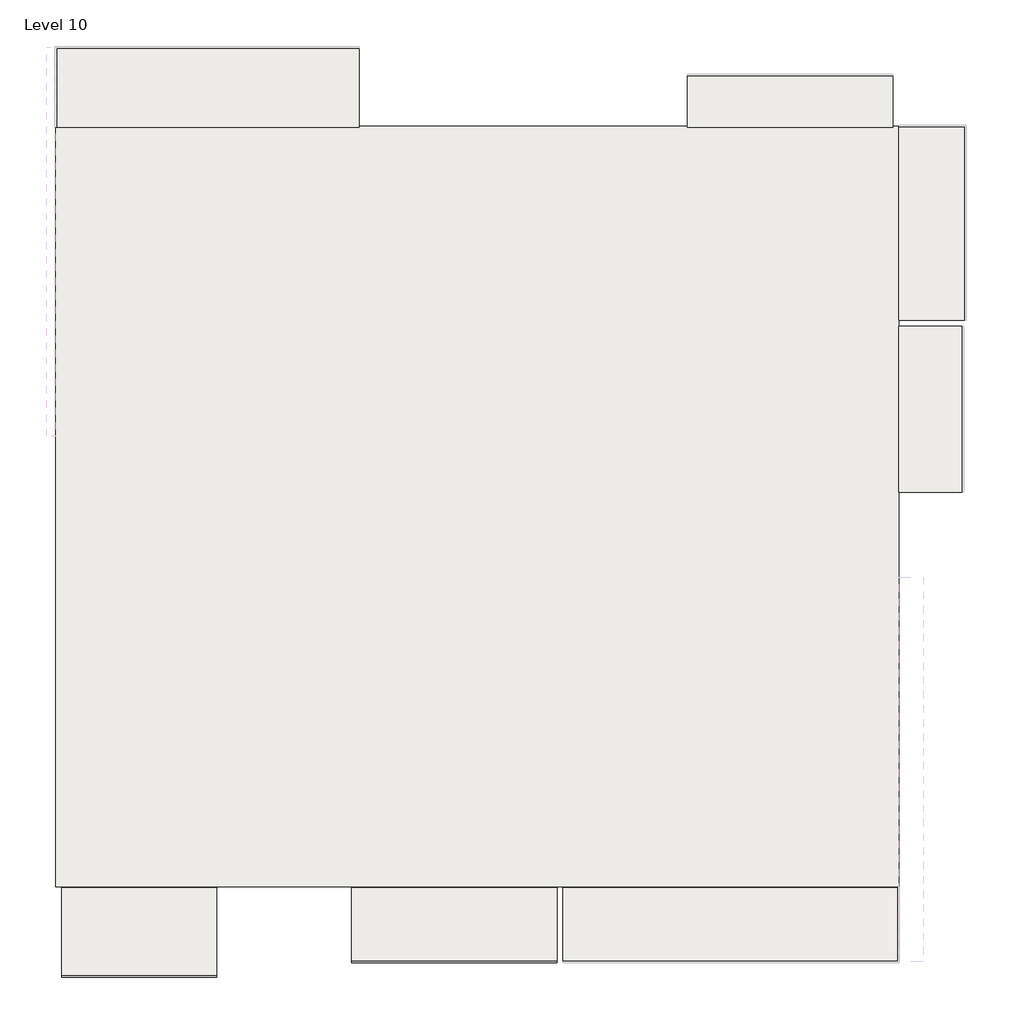
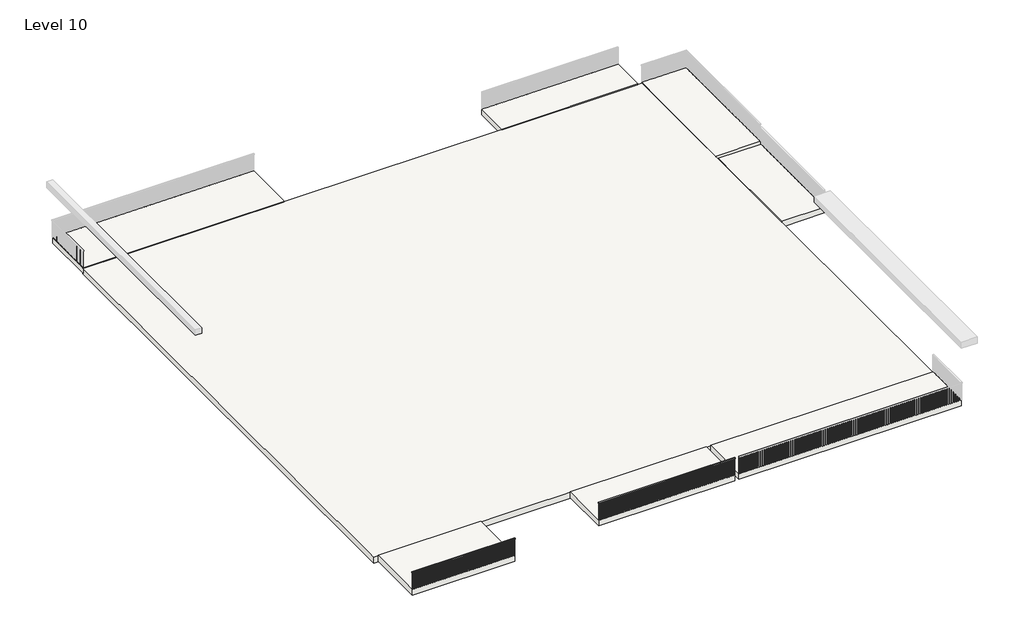
# One storey, part 1 of 5: 9 slabs, 2 railings.
"""IFC4 building model written with IfcOpenShell, lengths in millimetres."""

from ifc_helpers import new_model, si_unit, frame, origin, place, context, project, spatial, polyline, outline, extrude, element, save

model = new_model("IFC4")

# Units and contexts
model_context = context("Model", 3, world=origin())
ifc_project = project(units=[si_unit("LENGTHUNIT", "METRE", prefix="MILLI")], contexts=[model_context])

# Site, building, storey
site = spatial("IfcSite", under=ifc_project)
building = spatial("IfcBuilding", under=site)
storey = spatial("IfcBuildingStorey", under=building, Name="Level 10", Elevation=12496.8)

# Railings
placement = place(None, origin())
element("IfcRailing", 1, ObjectType="Handrail - Rectangular", at=placement, inside=storey, context=model_context, shape_type="SweptSolid", body=[
    extrude(outline(polyline([(-13630.2638778, -13399.9762475), (-13630.2638778, -13349.1762475), (-8499.4638778, -13349.1762475), (-8499.4638778, -13399.9762475), (-13630.2638778, -13399.9762475)])), frame((0.0, 0.0, 13360.4), z_axis=(0.0, 0.0, 1.0), x_axis=(1.0, 0.0, 0.0)), (0.0, 0.0, 1.0), 50.8),
    extrude(outline(polyline([(-8559.7888778, -13384.1012475), (-8559.7888778, -13365.0512475), (-8540.7388778, -13365.0512475), (-8540.7388778, -13384.1012475), (-8559.7888778, -13384.1012475)])), frame((0.0, 0.0, 12496.8), z_axis=(0.0, 0.0, 1.0), x_axis=(1.0, 0.0, 0.0)), (0.0, 0.0, 1.0), 863.6),
    extrude(outline(polyline([(-8661.3888778, -13384.1012475), (-8661.3888778, -13365.0512475), (-8642.3388778, -13365.0512475), (-8642.3388778, -13384.1012475), (-8661.3888778, -13384.1012475)])), frame((0.0, 0.0, 12496.8), z_axis=(0.0, 0.0, 1.0), x_axis=(1.0, 0.0, 0.0)), (0.0, 0.0, 1.0), 863.6),
    extrude(outline(polyline([(-8762.9888778, -13384.1012475), (-8762.9888778, -13365.0512475), (-8743.9388778, -13365.0512475), (-8743.9388778, -13384.1012475), (-8762.9888778, -13384.1012475)])), frame((0.0, 0.0, 12496.8), z_axis=(0.0, 0.0, 1.0), x_axis=(1.0, 0.0, 0.0)), (0.0, 0.0, 1.0), 863.6),
    extrude(outline(polyline([(-8864.5888778, -13384.1012475), (-8864.5888778, -13365.0512475), (-8845.5388778, -13365.0512475), (-8845.5388778, -13384.1012475), (-8864.5888778, -13384.1012475)])), frame((0.0, 0.0, 12496.8), z_axis=(0.0, 0.0, 1.0), x_axis=(1.0, 0.0, 0.0)), (0.0, 0.0, 1.0), 863.6),
    extrude(outline(polyline([(-8966.1888778, -13384.1012475), (-8966.1888778, -13365.0512475), (-8947.1388778, -13365.0512475), (-8947.1388778, -13384.1012475), (-8966.1888778, -13384.1012475)])), frame((0.0, 0.0, 12496.8), z_axis=(0.0, 0.0, 1.0), x_axis=(1.0, 0.0, 0.0)), (0.0, 0.0, 1.0), 863.6),
    extrude(outline(polyline([(-9067.7888778, -13384.1012475), (-9067.7888778, -13365.0512475), (-9048.7388778, -13365.0512475), (-9048.7388778, -13384.1012475), (-9067.7888778, -13384.1012475)])), frame((0.0, 0.0, 12496.8), z_axis=(0.0, 0.0, 1.0), x_axis=(1.0, 0.0, 0.0)), (0.0, 0.0, 1.0), 863.6),
    extrude(outline(polyline([(-9169.3888778, -13384.1012475), (-9169.3888778, -13365.0512475), (-9150.3388778, -13365.0512475), (-9150.3388778, -13384.1012475), (-9169.3888778, -13384.1012475)])), frame((0.0, 0.0, 12496.8), z_axis=(0.0, 0.0, 1.0), x_axis=(1.0, 0.0, 0.0)), (0.0, 0.0, 1.0), 863.6),
    extrude(outline(polyline([(-9270.9888778, -13384.1012475), (-9270.9888778, -13365.0512475), (-9251.9388778, -13365.0512475), (-9251.9388778, -13384.1012475), (-9270.9888778, -13384.1012475)])), frame((0.0, 0.0, 12496.8), z_axis=(0.0, 0.0, 1.0), x_axis=(1.0, 0.0, 0.0)), (0.0, 0.0, 1.0), 863.6),
    extrude(outline(polyline([(-9372.5888778, -13384.1012475), (-9372.5888778, -13365.0512475), (-9353.5388778, -13365.0512475), (-9353.5388778, -13384.1012475), (-9372.5888778, -13384.1012475)])), frame((0.0, 0.0, 12496.8), z_axis=(0.0, 0.0, 1.0), x_axis=(1.0, 0.0, 0.0)), (0.0, 0.0, 1.0), 863.6),
    extrude(outline(polyline([(-9474.1888778, -13384.1012475), (-9474.1888778, -13365.0512475), (-9455.1388778, -13365.0512475), (-9455.1388778, -13384.1012475), (-9474.1888778, -13384.1012475)])), frame((0.0, 0.0, 12496.8), z_axis=(0.0, 0.0, 1.0), x_axis=(1.0, 0.0, 0.0)), (0.0, 0.0, 1.0), 863.6),
    extrude(outline(polyline([(-9575.7888778, -13384.1012475), (-9575.7888778, -13365.0512475), (-9556.7388778, -13365.0512475), (-9556.7388778, -13384.1012475), (-9575.7888778, -13384.1012475)])), frame((0.0, 0.0, 12496.8), z_axis=(0.0, 0.0, 1.0), x_axis=(1.0, 0.0, 0.0)), (0.0, 0.0, 1.0), 863.6),
    extrude(outline(polyline([(-9677.3888778, -13384.1012475), (-9677.3888778, -13365.0512475), (-9658.3388778, -13365.0512475), (-9658.3388778, -13384.1012475), (-9677.3888778, -13384.1012475)])), frame((0.0, 0.0, 12496.8), z_axis=(0.0, 0.0, 1.0), x_axis=(1.0, 0.0, 0.0)), (0.0, 0.0, 1.0), 863.6),
    extrude(outline(polyline([(-9778.9888778, -13384.1012475), (-9778.9888778, -13365.0512475), (-9759.9388778, -13365.0512475), (-9759.9388778, -13384.1012475), (-9778.9888778, -13384.1012475)])), frame((0.0, 0.0, 12496.8), z_axis=(0.0, 0.0, 1.0), x_axis=(1.0, 0.0, 0.0)), (0.0, 0.0, 1.0), 863.6),
    extrude(outline(polyline([(-9880.5888778, -13384.1012475), (-9880.5888778, -13365.0512475), (-9861.5388778, -13365.0512475), (-9861.5388778, -13384.1012475), (-9880.5888778, -13384.1012475)])), frame((0.0, 0.0, 12496.8), z_axis=(0.0, 0.0, 1.0), x_axis=(1.0, 0.0, 0.0)), (0.0, 0.0, 1.0), 863.6),
    extrude(outline(polyline([(-9982.1888778, -13384.1012475), (-9982.1888778, -13365.0512475), (-9963.1388778, -13365.0512475), (-9963.1388778, -13384.1012475), (-9982.1888778, -13384.1012475)])), frame((0.0, 0.0, 12496.8), z_axis=(0.0, 0.0, 1.0), x_axis=(1.0, 0.0, 0.0)), (0.0, 0.0, 1.0), 863.6),
    extrude(outline(polyline([(-10083.7888778, -13384.1012475), (-10083.7888778, -13365.0512475), (-10064.7388778, -13365.0512475), (-10064.7388778, -13384.1012475), (-10083.7888778, -13384.1012475)])), frame((0.0, 0.0, 12496.8), z_axis=(0.0, 0.0, 1.0), x_axis=(1.0, 0.0, 0.0)), (0.0, 0.0, 1.0), 863.6),
    extrude(outline(polyline([(-10185.3888778, -13384.1012475), (-10185.3888778, -13365.0512475), (-10166.3388778, -13365.0512475), (-10166.3388778, -13384.1012475), (-10185.3888778, -13384.1012475)])), frame((0.0, 0.0, 12496.8), z_axis=(0.0, 0.0, 1.0), x_axis=(1.0, 0.0, 0.0)), (0.0, 0.0, 1.0), 863.6),
    extrude(outline(polyline([(-10286.9888778, -13384.1012475), (-10286.9888778, -13365.0512475), (-10267.9388778, -13365.0512475), (-10267.9388778, -13384.1012475), (-10286.9888778, -13384.1012475)])), frame((0.0, 0.0, 12496.8), z_axis=(0.0, 0.0, 1.0), x_axis=(1.0, 0.0, 0.0)), (0.0, 0.0, 1.0), 863.6),
    extrude(outline(polyline([(-10388.5888778, -13384.1012475), (-10388.5888778, -13365.0512475), (-10369.5388778, -13365.0512475), (-10369.5388778, -13384.1012475), (-10388.5888778, -13384.1012475)])), frame((0.0, 0.0, 12496.8), z_axis=(0.0, 0.0, 1.0), x_axis=(1.0, 0.0, 0.0)), (0.0, 0.0, 1.0), 863.6),
    extrude(outline(polyline([(-10490.1888778, -13384.1012475), (-10490.1888778, -13365.0512475), (-10471.1388778, -13365.0512475), (-10471.1388778, -13384.1012475), (-10490.1888778, -13384.1012475)])), frame((0.0, 0.0, 12496.8), z_axis=(0.0, 0.0, 1.0), x_axis=(1.0, 0.0, 0.0)), (0.0, 0.0, 1.0), 863.6),
    extrude(outline(polyline([(-10591.7888778, -13384.1012475), (-10591.7888778, -13365.0512475), (-10572.7388778, -13365.0512475), (-10572.7388778, -13384.1012475), (-10591.7888778, -13384.1012475)])), frame((0.0, 0.0, 12496.8), z_axis=(0.0, 0.0, 1.0), x_axis=(1.0, 0.0, 0.0)), (0.0, 0.0, 1.0), 863.6),
    extrude(outline(polyline([(-10693.3888778, -13384.1012475), (-10693.3888778, -13365.0512475), (-10674.3388778, -13365.0512475), (-10674.3388778, -13384.1012475), (-10693.3888778, -13384.1012475)])), frame((0.0, 0.0, 12496.8), z_axis=(0.0, 0.0, 1.0), x_axis=(1.0, 0.0, 0.0)), (0.0, 0.0, 1.0), 863.6),
    extrude(outline(polyline([(-10794.9888778, -13384.1012475), (-10794.9888778, -13365.0512475), (-10775.9388778, -13365.0512475), (-10775.9388778, -13384.1012475), (-10794.9888778, -13384.1012475)])), frame((0.0, 0.0, 12496.8), z_axis=(0.0, 0.0, 1.0), x_axis=(1.0, 0.0, 0.0)), (0.0, 0.0, 1.0), 863.6),
    extrude(outline(polyline([(-10896.5888778, -13384.1012475), (-10896.5888778, -13365.0512475), (-10877.5388778, -13365.0512475), (-10877.5388778, -13384.1012475), (-10896.5888778, -13384.1012475)])), frame((0.0, 0.0, 12496.8), z_axis=(0.0, 0.0, 1.0), x_axis=(1.0, 0.0, 0.0)), (0.0, 0.0, 1.0), 863.6),
    extrude(outline(polyline([(-10998.1888778, -13384.1012475), (-10998.1888778, -13365.0512475), (-10979.1388778, -13365.0512475), (-10979.1388778, -13384.1012475), (-10998.1888778, -13384.1012475)])), frame((0.0, 0.0, 12496.8), z_axis=(0.0, 0.0, 1.0), x_axis=(1.0, 0.0, 0.0)), (0.0, 0.0, 1.0), 863.6),
    extrude(outline(polyline([(-11099.7888778, -13384.1012475), (-11099.7888778, -13365.0512475), (-11080.7388778, -13365.0512475), (-11080.7388778, -13384.1012475), (-11099.7888778, -13384.1012475)])), frame((0.0, 0.0, 12496.8), z_axis=(0.0, 0.0, 1.0), x_axis=(1.0, 0.0, 0.0)), (0.0, 0.0, 1.0), 863.6),
    extrude(outline(polyline([(-11201.3888778, -13384.1012475), (-11201.3888778, -13365.0512475), (-11182.3388778, -13365.0512475), (-11182.3388778, -13384.1012475), (-11201.3888778, -13384.1012475)])), frame((0.0, 0.0, 12496.8), z_axis=(0.0, 0.0, 1.0), x_axis=(1.0, 0.0, 0.0)), (0.0, 0.0, 1.0), 863.6),
    extrude(outline(polyline([(-11302.9888778, -13384.1012475), (-11302.9888778, -13365.0512475), (-11283.9388778, -13365.0512475), (-11283.9388778, -13384.1012475), (-11302.9888778, -13384.1012475)])), frame((0.0, 0.0, 12496.8), z_axis=(0.0, 0.0, 1.0), x_axis=(1.0, 0.0, 0.0)), (0.0, 0.0, 1.0), 863.6),
    extrude(outline(polyline([(-11404.5888778, -13384.1012475), (-11404.5888778, -13365.0512475), (-11385.5388778, -13365.0512475), (-11385.5388778, -13384.1012475), (-11404.5888778, -13384.1012475)])), frame((0.0, 0.0, 12496.8), z_axis=(0.0, 0.0, 1.0), x_axis=(1.0, 0.0, 0.0)), (0.0, 0.0, 1.0), 863.6),
    extrude(outline(polyline([(-11506.1888778, -13384.1012475), (-11506.1888778, -13365.0512475), (-11487.1388778, -13365.0512475), (-11487.1388778, -13384.1012475), (-11506.1888778, -13384.1012475)])), frame((0.0, 0.0, 12496.8), z_axis=(0.0, 0.0, 1.0), x_axis=(1.0, 0.0, 0.0)), (0.0, 0.0, 1.0), 863.6),
    extrude(outline(polyline([(-11607.7888778, -13384.1012475), (-11607.7888778, -13365.0512475), (-11588.7388778, -13365.0512475), (-11588.7388778, -13384.1012475), (-11607.7888778, -13384.1012475)])), frame((0.0, 0.0, 12496.8), z_axis=(0.0, 0.0, 1.0), x_axis=(1.0, 0.0, 0.0)), (0.0, 0.0, 1.0), 863.6),
    extrude(outline(polyline([(-11709.3888778, -13384.1012475), (-11709.3888778, -13365.0512475), (-11690.3388778, -13365.0512475), (-11690.3388778, -13384.1012475), (-11709.3888778, -13384.1012475)])), frame((0.0, 0.0, 12496.8), z_axis=(0.0, 0.0, 1.0), x_axis=(1.0, 0.0, 0.0)), (0.0, 0.0, 1.0), 863.6),
    extrude(outline(polyline([(-11810.9888778, -13384.1012475), (-11810.9888778, -13365.0512475), (-11791.9388778, -13365.0512475), (-11791.9388778, -13384.1012475), (-11810.9888778, -13384.1012475)])), frame((0.0, 0.0, 12496.8), z_axis=(0.0, 0.0, 1.0), x_axis=(1.0, 0.0, 0.0)), (0.0, 0.0, 1.0), 863.6),
    extrude(outline(polyline([(-11912.5888778, -13384.1012475), (-11912.5888778, -13365.0512475), (-11893.5388778, -13365.0512475), (-11893.5388778, -13384.1012475), (-11912.5888778, -13384.1012475)])), frame((0.0, 0.0, 12496.8), z_axis=(0.0, 0.0, 1.0), x_axis=(1.0, 0.0, 0.0)), (0.0, 0.0, 1.0), 863.6),
    extrude(outline(polyline([(-12014.1888778, -13384.1012475), (-12014.1888778, -13365.0512475), (-11995.1388778, -13365.0512475), (-11995.1388778, -13384.1012475), (-12014.1888778, -13384.1012475)])), frame((0.0, 0.0, 12496.8), z_axis=(0.0, 0.0, 1.0), x_axis=(1.0, 0.0, 0.0)), (0.0, 0.0, 1.0), 863.6),
    extrude(outline(polyline([(-12115.7888778, -13384.1012475), (-12115.7888778, -13365.0512475), (-12096.7388778, -13365.0512475), (-12096.7388778, -13384.1012475), (-12115.7888778, -13384.1012475)])), frame((0.0, 0.0, 12496.8), z_axis=(0.0, 0.0, 1.0), x_axis=(1.0, 0.0, 0.0)), (0.0, 0.0, 1.0), 863.6),
    extrude(outline(polyline([(-12217.3888778, -13384.1012475), (-12217.3888778, -13365.0512475), (-12198.3388778, -13365.0512475), (-12198.3388778, -13384.1012475), (-12217.3888778, -13384.1012475)])), frame((0.0, 0.0, 12496.8), z_axis=(0.0, 0.0, 1.0), x_axis=(1.0, 0.0, 0.0)), (0.0, 0.0, 1.0), 863.6),
    extrude(outline(polyline([(-12318.9888778, -13384.1012475), (-12318.9888778, -13365.0512475), (-12299.9388778, -13365.0512475), (-12299.9388778, -13384.1012475), (-12318.9888778, -13384.1012475)])), frame((0.0, 0.0, 12496.8), z_axis=(0.0, 0.0, 1.0), x_axis=(1.0, 0.0, 0.0)), (0.0, 0.0, 1.0), 863.6),
    extrude(outline(polyline([(-12420.5888778, -13384.1012475), (-12420.5888778, -13365.0512475), (-12401.5388778, -13365.0512475), (-12401.5388778, -13384.1012475), (-12420.5888778, -13384.1012475)])), frame((0.0, 0.0, 12496.8), z_axis=(0.0, 0.0, 1.0), x_axis=(1.0, 0.0, 0.0)), (0.0, 0.0, 1.0), 863.6),
    extrude(outline(polyline([(-12522.1888778, -13384.1012475), (-12522.1888778, -13365.0512475), (-12503.1388778, -13365.0512475), (-12503.1388778, -13384.1012475), (-12522.1888778, -13384.1012475)])), frame((0.0, 0.0, 12496.8), z_axis=(0.0, 0.0, 1.0), x_axis=(1.0, 0.0, 0.0)), (0.0, 0.0, 1.0), 863.6),
    extrude(outline(polyline([(-12623.7888778, -13384.1012475), (-12623.7888778, -13365.0512475), (-12604.7388778, -13365.0512475), (-12604.7388778, -13384.1012475), (-12623.7888778, -13384.1012475)])), frame((0.0, 0.0, 12496.8), z_axis=(0.0, 0.0, 1.0), x_axis=(1.0, 0.0, 0.0)), (0.0, 0.0, 1.0), 863.6),
    extrude(outline(polyline([(-12725.3888778, -13384.1012475), (-12725.3888778, -13365.0512475), (-12706.3388778, -13365.0512475), (-12706.3388778, -13384.1012475), (-12725.3888778, -13384.1012475)])), frame((0.0, 0.0, 12496.8), z_axis=(0.0, 0.0, 1.0), x_axis=(1.0, 0.0, 0.0)), (0.0, 0.0, 1.0), 863.6),
    extrude(outline(polyline([(-12826.9888778, -13384.1012475), (-12826.9888778, -13365.0512475), (-12807.9388778, -13365.0512475), (-12807.9388778, -13384.1012475), (-12826.9888778, -13384.1012475)])), frame((0.0, 0.0, 12496.8), z_axis=(0.0, 0.0, 1.0), x_axis=(1.0, 0.0, 0.0)), (0.0, 0.0, 1.0), 863.6),
    extrude(outline(polyline([(-12928.5888778, -13384.1012475), (-12928.5888778, -13365.0512475), (-12909.5388778, -13365.0512475), (-12909.5388778, -13384.1012475), (-12928.5888778, -13384.1012475)])), frame((0.0, 0.0, 12496.8), z_axis=(0.0, 0.0, 1.0), x_axis=(1.0, 0.0, 0.0)), (0.0, 0.0, 1.0), 863.6),
    extrude(outline(polyline([(-13030.1888778, -13384.1012475), (-13030.1888778, -13365.0512475), (-13011.1388778, -13365.0512475), (-13011.1388778, -13384.1012475), (-13030.1888778, -13384.1012475)])), frame((0.0, 0.0, 12496.8), z_axis=(0.0, 0.0, 1.0), x_axis=(1.0, 0.0, 0.0)), (0.0, 0.0, 1.0), 863.6),
    extrude(outline(polyline([(-13131.7888778, -13384.1012475), (-13131.7888778, -13365.0512475), (-13112.7388778, -13365.0512475), (-13112.7388778, -13384.1012475), (-13131.7888778, -13384.1012475)])), frame((0.0, 0.0, 12496.8), z_axis=(0.0, 0.0, 1.0), x_axis=(1.0, 0.0, 0.0)), (0.0, 0.0, 1.0), 863.6),
    extrude(outline(polyline([(-13233.3888778, -13384.1012475), (-13233.3888778, -13365.0512475), (-13214.3388778, -13365.0512475), (-13214.3388778, -13384.1012475), (-13233.3888778, -13384.1012475)])), frame((0.0, 0.0, 12496.8), z_axis=(0.0, 0.0, 1.0), x_axis=(1.0, 0.0, 0.0)), (0.0, 0.0, 1.0), 863.6),
    extrude(outline(polyline([(-13334.9888778, -13384.1012475), (-13334.9888778, -13365.0512475), (-13315.9388778, -13365.0512475), (-13315.9388778, -13384.1012475), (-13334.9888778, -13384.1012475)])), frame((0.0, 0.0, 12496.8), z_axis=(0.0, 0.0, 1.0), x_axis=(1.0, 0.0, 0.0)), (0.0, 0.0, 1.0), 863.6),
    extrude(outline(polyline([(-13436.5888778, -13384.1012475), (-13436.5888778, -13365.0512475), (-13417.5388778, -13365.0512475), (-13417.5388778, -13384.1012475), (-13436.5888778, -13384.1012475)])), frame((0.0, 0.0, 12496.8), z_axis=(0.0, 0.0, 1.0), x_axis=(1.0, 0.0, 0.0)), (0.0, 0.0, 1.0), 863.6),
    extrude(outline(polyline([(-13538.1888778, -13384.1012475), (-13538.1888778, -13365.0512475), (-13519.1388778, -13365.0512475), (-13519.1388778, -13384.1012475), (-13538.1888778, -13384.1012475)])), frame((0.0, 0.0, 12496.8), z_axis=(0.0, 0.0, 1.0), x_axis=(1.0, 0.0, 0.0)), (0.0, 0.0, 1.0), 863.6),
    extrude(outline(polyline([(-8518.5138778, -13384.1012475), (-8518.5138778, -13365.0512475), (-8499.4638778, -13365.0512475), (-8499.4638778, -13384.1012475), (-8518.5138778, -13384.1012475)])), frame((0.0, 0.0, 12496.8), z_axis=(0.0, 0.0, 1.0), x_axis=(1.0, 0.0, 0.0)), (0.0, 0.0, 1.0), 863.6),
    extrude(outline(polyline([(-13630.2638778, -13384.1012475), (-13630.2638778, -13365.0512475), (-13611.2138778, -13365.0512475), (-13611.2138778, -13384.1012475), (-13630.2638778, -13384.1012475)])), frame((0.0, 0.0, 12496.8), z_axis=(0.0, 0.0, 1.0), x_axis=(1.0, 0.0, 0.0)), (0.0, 0.0, 1.0), 863.6),
])
element("IfcRailing", 2, ObjectType="Handrail - Rectangular", at=placement, inside=storey, context=model_context, shape_type="SweptSolid", body=[
    extrude(outline(polyline([(-4029.0638778, -12911.7749501), (-4029.0638778, -12860.9749501), (2778.1361222, -12860.9749501), (2778.1361222, -12911.7749501), (-4029.0638778, -12911.7749501)])), frame((0.0, 0.0, 13360.4), z_axis=(0.0, 0.0, 1.0), x_axis=(1.0, 0.0, 0.0)), (0.0, 0.0, 1.0), 50.8),
    extrude(outline(polyline([(2667.0111222, -12895.8999501), (2667.0111222, -12876.8499501), (2686.0611222, -12876.8499501), (2686.0611222, -12895.8999501), (2667.0111222, -12895.8999501)])), frame((0.0, 0.0, 12496.8), z_axis=(0.0, 0.0, 1.0), x_axis=(1.0, 0.0, 0.0)), (0.0, 0.0, 1.0), 863.6),
    extrude(outline(polyline([(2565.4111222, -12895.8999501), (2565.4111222, -12876.8499501), (2584.4611222, -12876.8499501), (2584.4611222, -12895.8999501), (2565.4111222, -12895.8999501)])), frame((0.0, 0.0, 12496.8), z_axis=(0.0, 0.0, 1.0), x_axis=(1.0, 0.0, 0.0)), (0.0, 0.0, 1.0), 863.6),
    extrude(outline(polyline([(2463.8111222, -12895.8999501), (2463.8111222, -12876.8499501), (2482.8611222, -12876.8499501), (2482.8611222, -12895.8999501), (2463.8111222, -12895.8999501)])), frame((0.0, 0.0, 12496.8), z_axis=(0.0, 0.0, 1.0), x_axis=(1.0, 0.0, 0.0)), (0.0, 0.0, 1.0), 863.6),
    extrude(outline(polyline([(2362.2111222, -12895.8999501), (2362.2111222, -12876.8499501), (2381.2611222, -12876.8499501), (2381.2611222, -12895.8999501), (2362.2111222, -12895.8999501)])), frame((0.0, 0.0, 12496.8), z_axis=(0.0, 0.0, 1.0), x_axis=(1.0, 0.0, 0.0)), (0.0, 0.0, 1.0), 863.6),
    extrude(outline(polyline([(2260.6111222, -12895.8999501), (2260.6111222, -12876.8499501), (2279.6611222, -12876.8499501), (2279.6611222, -12895.8999501), (2260.6111222, -12895.8999501)])), frame((0.0, 0.0, 12496.8), z_axis=(0.0, 0.0, 1.0), x_axis=(1.0, 0.0, 0.0)), (0.0, 0.0, 1.0), 863.6),
    extrude(outline(polyline([(2159.0111222, -12895.8999501), (2159.0111222, -12876.8499501), (2178.0611222, -12876.8499501), (2178.0611222, -12895.8999501), (2159.0111222, -12895.8999501)])), frame((0.0, 0.0, 12496.8), z_axis=(0.0, 0.0, 1.0), x_axis=(1.0, 0.0, 0.0)), (0.0, 0.0, 1.0), 863.6),
    extrude(outline(polyline([(2057.4111222, -12895.8999501), (2057.4111222, -12876.8499501), (2076.4611222, -12876.8499501), (2076.4611222, -12895.8999501), (2057.4111222, -12895.8999501)])), frame((0.0, 0.0, 12496.8), z_axis=(0.0, 0.0, 1.0), x_axis=(1.0, 0.0, 0.0)), (0.0, 0.0, 1.0), 863.6),
    extrude(outline(polyline([(1955.8111222, -12895.8999501), (1955.8111222, -12876.8499501), (1974.8611222, -12876.8499501), (1974.8611222, -12895.8999501), (1955.8111222, -12895.8999501)])), frame((0.0, 0.0, 12496.8), z_axis=(0.0, 0.0, 1.0), x_axis=(1.0, 0.0, 0.0)), (0.0, 0.0, 1.0), 863.6),
    extrude(outline(polyline([(1854.2111222, -12895.8999501), (1854.2111222, -12876.8499501), (1873.2611222, -12876.8499501), (1873.2611222, -12895.8999501), (1854.2111222, -12895.8999501)])), frame((0.0, 0.0, 12496.8), z_axis=(0.0, 0.0, 1.0), x_axis=(1.0, 0.0, 0.0)), (0.0, 0.0, 1.0), 863.6),
    extrude(outline(polyline([(1752.6111222, -12895.8999501), (1752.6111222, -12876.8499501), (1771.6611222, -12876.8499501), (1771.6611222, -12895.8999501), (1752.6111222, -12895.8999501)])), frame((0.0, 0.0, 12496.8), z_axis=(0.0, 0.0, 1.0), x_axis=(1.0, 0.0, 0.0)), (0.0, 0.0, 1.0), 863.6),
    extrude(outline(polyline([(1651.0111222, -12895.8999501), (1651.0111222, -12876.8499501), (1670.0611222, -12876.8499501), (1670.0611222, -12895.8999501), (1651.0111222, -12895.8999501)])), frame((0.0, 0.0, 12496.8), z_axis=(0.0, 0.0, 1.0), x_axis=(1.0, 0.0, 0.0)), (0.0, 0.0, 1.0), 863.6),
    extrude(outline(polyline([(1549.4111222, -12895.8999501), (1549.4111222, -12876.8499501), (1568.4611222, -12876.8499501), (1568.4611222, -12895.8999501), (1549.4111222, -12895.8999501)])), frame((0.0, 0.0, 12496.8), z_axis=(0.0, 0.0, 1.0), x_axis=(1.0, 0.0, 0.0)), (0.0, 0.0, 1.0), 863.6),
    extrude(outline(polyline([(1447.8111222, -12895.8999501), (1447.8111222, -12876.8499501), (1466.8611222, -12876.8499501), (1466.8611222, -12895.8999501), (1447.8111222, -12895.8999501)])), frame((0.0, 0.0, 12496.8), z_axis=(0.0, 0.0, 1.0), x_axis=(1.0, 0.0, 0.0)), (0.0, 0.0, 1.0), 863.6),
    extrude(outline(polyline([(1346.2111222, -12895.8999501), (1346.2111222, -12876.8499501), (1365.2611222, -12876.8499501), (1365.2611222, -12895.8999501), (1346.2111222, -12895.8999501)])), frame((0.0, 0.0, 12496.8), z_axis=(0.0, 0.0, 1.0), x_axis=(1.0, 0.0, 0.0)), (0.0, 0.0, 1.0), 863.6),
    extrude(outline(polyline([(1244.6111222, -12895.8999501), (1244.6111222, -12876.8499501), (1263.6611222, -12876.8499501), (1263.6611222, -12895.8999501), (1244.6111222, -12895.8999501)])), frame((0.0, 0.0, 12496.8), z_axis=(0.0, 0.0, 1.0), x_axis=(1.0, 0.0, 0.0)), (0.0, 0.0, 1.0), 863.6),
    extrude(outline(polyline([(1143.0111222, -12895.8999501), (1143.0111222, -12876.8499501), (1162.0611222, -12876.8499501), (1162.0611222, -12895.8999501), (1143.0111222, -12895.8999501)])), frame((0.0, 0.0, 12496.8), z_axis=(0.0, 0.0, 1.0), x_axis=(1.0, 0.0, 0.0)), (0.0, 0.0, 1.0), 863.6),
    extrude(outline(polyline([(1041.4111222, -12895.8999501), (1041.4111222, -12876.8499501), (1060.4611222, -12876.8499501), (1060.4611222, -12895.8999501), (1041.4111222, -12895.8999501)])), frame((0.0, 0.0, 12496.8), z_axis=(0.0, 0.0, 1.0), x_axis=(1.0, 0.0, 0.0)), (0.0, 0.0, 1.0), 863.6),
    extrude(outline(polyline([(939.8111222, -12895.8999501), (939.8111222, -12876.8499501), (958.8611222, -12876.8499501), (958.8611222, -12895.8999501), (939.8111222, -12895.8999501)])), frame((0.0, 0.0, 12496.8), z_axis=(0.0, 0.0, 1.0), x_axis=(1.0, 0.0, 0.0)), (0.0, 0.0, 1.0), 863.6),
    extrude(outline(polyline([(838.2111222, -12895.8999501), (838.2111222, -12876.8499501), (857.2611222, -12876.8499501), (857.2611222, -12895.8999501), (838.2111222, -12895.8999501)])), frame((0.0, 0.0, 12496.8), z_axis=(0.0, 0.0, 1.0), x_axis=(1.0, 0.0, 0.0)), (0.0, 0.0, 1.0), 863.6),
    extrude(outline(polyline([(736.6111222, -12895.8999501), (736.6111222, -12876.8499501), (755.6611222, -12876.8499501), (755.6611222, -12895.8999501), (736.6111222, -12895.8999501)])), frame((0.0, 0.0, 12496.8), z_axis=(0.0, 0.0, 1.0), x_axis=(1.0, 0.0, 0.0)), (0.0, 0.0, 1.0), 863.6),
    extrude(outline(polyline([(635.0111222, -12895.8999501), (635.0111222, -12876.8499501), (654.0611222, -12876.8499501), (654.0611222, -12895.8999501), (635.0111222, -12895.8999501)])), frame((0.0, 0.0, 12496.8), z_axis=(0.0, 0.0, 1.0), x_axis=(1.0, 0.0, 0.0)), (0.0, 0.0, 1.0), 863.6),
    extrude(outline(polyline([(533.4111222, -12895.8999501), (533.4111222, -12876.8499501), (552.4611222, -12876.8499501), (552.4611222, -12895.8999501), (533.4111222, -12895.8999501)])), frame((0.0, 0.0, 12496.8), z_axis=(0.0, 0.0, 1.0), x_axis=(1.0, 0.0, 0.0)), (0.0, 0.0, 1.0), 863.6),
    extrude(outline(polyline([(431.8111222, -12895.8999501), (431.8111222, -12876.8499501), (450.8611222, -12876.8499501), (450.8611222, -12895.8999501), (431.8111222, -12895.8999501)])), frame((0.0, 0.0, 12496.8), z_axis=(0.0, 0.0, 1.0), x_axis=(1.0, 0.0, 0.0)), (0.0, 0.0, 1.0), 863.6),
    extrude(outline(polyline([(330.2111222, -12895.8999501), (330.2111222, -12876.8499501), (349.2611222, -12876.8499501), (349.2611222, -12895.8999501), (330.2111222, -12895.8999501)])), frame((0.0, 0.0, 12496.8), z_axis=(0.0, 0.0, 1.0), x_axis=(1.0, 0.0, 0.0)), (0.0, 0.0, 1.0), 863.6),
    extrude(outline(polyline([(228.6111222, -12895.8999501), (228.6111222, -12876.8499501), (247.6611222, -12876.8499501), (247.6611222, -12895.8999501), (228.6111222, -12895.8999501)])), frame((0.0, 0.0, 12496.8), z_axis=(0.0, 0.0, 1.0), x_axis=(1.0, 0.0, 0.0)), (0.0, 0.0, 1.0), 863.6),
    extrude(outline(polyline([(127.0111222, -12895.8999501), (127.0111222, -12876.8499501), (146.0611222, -12876.8499501), (146.0611222, -12895.8999501), (127.0111222, -12895.8999501)])), frame((0.0, 0.0, 12496.8), z_axis=(0.0, 0.0, 1.0), x_axis=(1.0, 0.0, 0.0)), (0.0, 0.0, 1.0), 863.6),
    extrude(outline(polyline([(25.4111222, -12895.8999501), (25.4111222, -12876.8499501), (44.4611222, -12876.8499501), (44.4611222, -12895.8999501), (25.4111222, -12895.8999501)])), frame((0.0, 0.0, 12496.8), z_axis=(0.0, 0.0, 1.0), x_axis=(1.0, 0.0, 0.0)), (0.0, 0.0, 1.0), 863.6),
    extrude(outline(polyline([(-76.1888778, -12895.8999501), (-76.1888778, -12876.8499501), (-57.1388778, -12876.8499501), (-57.1388778, -12895.8999501), (-76.1888778, -12895.8999501)])), frame((0.0, 0.0, 12496.8), z_axis=(0.0, 0.0, 1.0), x_axis=(1.0, 0.0, 0.0)), (0.0, 0.0, 1.0), 863.6),
    extrude(outline(polyline([(-177.7888778, -12895.8999501), (-177.7888778, -12876.8499501), (-158.7388778, -12876.8499501), (-158.7388778, -12895.8999501), (-177.7888778, -12895.8999501)])), frame((0.0, 0.0, 12496.8), z_axis=(0.0, 0.0, 1.0), x_axis=(1.0, 0.0, 0.0)), (0.0, 0.0, 1.0), 863.6),
    extrude(outline(polyline([(-279.3888778, -12895.8999501), (-279.3888778, -12876.8499501), (-260.3388778, -12876.8499501), (-260.3388778, -12895.8999501), (-279.3888778, -12895.8999501)])), frame((0.0, 0.0, 12496.8), z_axis=(0.0, 0.0, 1.0), x_axis=(1.0, 0.0, 0.0)), (0.0, 0.0, 1.0), 863.6),
    extrude(outline(polyline([(-380.9888778, -12895.8999501), (-380.9888778, -12876.8499501), (-361.9388778, -12876.8499501), (-361.9388778, -12895.8999501), (-380.9888778, -12895.8999501)])), frame((0.0, 0.0, 12496.8), z_axis=(0.0, 0.0, 1.0), x_axis=(1.0, 0.0, 0.0)), (0.0, 0.0, 1.0), 863.6),
    extrude(outline(polyline([(-482.5888778, -12895.8999501), (-482.5888778, -12876.8499501), (-463.5388778, -12876.8499501), (-463.5388778, -12895.8999501), (-482.5888778, -12895.8999501)])), frame((0.0, 0.0, 12496.8), z_axis=(0.0, 0.0, 1.0), x_axis=(1.0, 0.0, 0.0)), (0.0, 0.0, 1.0), 863.6),
    extrude(outline(polyline([(-584.1888778, -12895.8999501), (-584.1888778, -12876.8499501), (-565.1388778, -12876.8499501), (-565.1388778, -12895.8999501), (-584.1888778, -12895.8999501)])), frame((0.0, 0.0, 12496.8), z_axis=(0.0, 0.0, 1.0), x_axis=(1.0, 0.0, 0.0)), (0.0, 0.0, 1.0), 863.6),
    extrude(outline(polyline([(-685.7888778, -12895.8999501), (-685.7888778, -12876.8499501), (-666.7388778, -12876.8499501), (-666.7388778, -12895.8999501), (-685.7888778, -12895.8999501)])), frame((0.0, 0.0, 12496.8), z_axis=(0.0, 0.0, 1.0), x_axis=(1.0, 0.0, 0.0)), (0.0, 0.0, 1.0), 863.6),
    extrude(outline(polyline([(-787.3888778, -12895.8999501), (-787.3888778, -12876.8499501), (-768.3388778, -12876.8499501), (-768.3388778, -12895.8999501), (-787.3888778, -12895.8999501)])), frame((0.0, 0.0, 12496.8), z_axis=(0.0, 0.0, 1.0), x_axis=(1.0, 0.0, 0.0)), (0.0, 0.0, 1.0), 863.6),
    extrude(outline(polyline([(-888.9888778, -12895.8999501), (-888.9888778, -12876.8499501), (-869.9388778, -12876.8499501), (-869.9388778, -12895.8999501), (-888.9888778, -12895.8999501)])), frame((0.0, 0.0, 12496.8), z_axis=(0.0, 0.0, 1.0), x_axis=(1.0, 0.0, 0.0)), (0.0, 0.0, 1.0), 863.6),
    extrude(outline(polyline([(-990.5888778, -12895.8999501), (-990.5888778, -12876.8499501), (-971.5388778, -12876.8499501), (-971.5388778, -12895.8999501), (-990.5888778, -12895.8999501)])), frame((0.0, 0.0, 12496.8), z_axis=(0.0, 0.0, 1.0), x_axis=(1.0, 0.0, 0.0)), (0.0, 0.0, 1.0), 863.6),
    extrude(outline(polyline([(-1092.1888778, -12895.8999501), (-1092.1888778, -12876.8499501), (-1073.1388778, -12876.8499501), (-1073.1388778, -12895.8999501), (-1092.1888778, -12895.8999501)])), frame((0.0, 0.0, 12496.8), z_axis=(0.0, 0.0, 1.0), x_axis=(1.0, 0.0, 0.0)), (0.0, 0.0, 1.0), 863.6),
    extrude(outline(polyline([(-1193.7888778, -12895.8999501), (-1193.7888778, -12876.8499501), (-1174.7388778, -12876.8499501), (-1174.7388778, -12895.8999501), (-1193.7888778, -12895.8999501)])), frame((0.0, 0.0, 12496.8), z_axis=(0.0, 0.0, 1.0), x_axis=(1.0, 0.0, 0.0)), (0.0, 0.0, 1.0), 863.6),
    extrude(outline(polyline([(-1295.3888778, -12895.8999501), (-1295.3888778, -12876.8499501), (-1276.3388778, -12876.8499501), (-1276.3388778, -12895.8999501), (-1295.3888778, -12895.8999501)])), frame((0.0, 0.0, 12496.8), z_axis=(0.0, 0.0, 1.0), x_axis=(1.0, 0.0, 0.0)), (0.0, 0.0, 1.0), 863.6),
    extrude(outline(polyline([(-1396.9888778, -12895.8999501), (-1396.9888778, -12876.8499501), (-1377.9388778, -12876.8499501), (-1377.9388778, -12895.8999501), (-1396.9888778, -12895.8999501)])), frame((0.0, 0.0, 12496.8), z_axis=(0.0, 0.0, 1.0), x_axis=(1.0, 0.0, 0.0)), (0.0, 0.0, 1.0), 863.6),
    extrude(outline(polyline([(-1498.5888778, -12895.8999501), (-1498.5888778, -12876.8499501), (-1479.5388778, -12876.8499501), (-1479.5388778, -12895.8999501), (-1498.5888778, -12895.8999501)])), frame((0.0, 0.0, 12496.8), z_axis=(0.0, 0.0, 1.0), x_axis=(1.0, 0.0, 0.0)), (0.0, 0.0, 1.0), 863.6),
    extrude(outline(polyline([(-1600.1888778, -12895.8999501), (-1600.1888778, -12876.8499501), (-1581.1388778, -12876.8499501), (-1581.1388778, -12895.8999501), (-1600.1888778, -12895.8999501)])), frame((0.0, 0.0, 12496.8), z_axis=(0.0, 0.0, 1.0), x_axis=(1.0, 0.0, 0.0)), (0.0, 0.0, 1.0), 863.6),
    extrude(outline(polyline([(-1701.7888778, -12895.8999501), (-1701.7888778, -12876.8499501), (-1682.7388778, -12876.8499501), (-1682.7388778, -12895.8999501), (-1701.7888778, -12895.8999501)])), frame((0.0, 0.0, 12496.8), z_axis=(0.0, 0.0, 1.0), x_axis=(1.0, 0.0, 0.0)), (0.0, 0.0, 1.0), 863.6),
    extrude(outline(polyline([(-1803.3888778, -12895.8999501), (-1803.3888778, -12876.8499501), (-1784.3388778, -12876.8499501), (-1784.3388778, -12895.8999501), (-1803.3888778, -12895.8999501)])), frame((0.0, 0.0, 12496.8), z_axis=(0.0, 0.0, 1.0), x_axis=(1.0, 0.0, 0.0)), (0.0, 0.0, 1.0), 863.6),
    extrude(outline(polyline([(-1904.9888778, -12895.8999501), (-1904.9888778, -12876.8499501), (-1885.9388778, -12876.8499501), (-1885.9388778, -12895.8999501), (-1904.9888778, -12895.8999501)])), frame((0.0, 0.0, 12496.8), z_axis=(0.0, 0.0, 1.0), x_axis=(1.0, 0.0, 0.0)), (0.0, 0.0, 1.0), 863.6),
    extrude(outline(polyline([(-2006.5888778, -12895.8999501), (-2006.5888778, -12876.8499501), (-1987.5388778, -12876.8499501), (-1987.5388778, -12895.8999501), (-2006.5888778, -12895.8999501)])), frame((0.0, 0.0, 12496.8), z_axis=(0.0, 0.0, 1.0), x_axis=(1.0, 0.0, 0.0)), (0.0, 0.0, 1.0), 863.6),
    extrude(outline(polyline([(-2108.1888778, -12895.8999501), (-2108.1888778, -12876.8499501), (-2089.1388778, -12876.8499501), (-2089.1388778, -12895.8999501), (-2108.1888778, -12895.8999501)])), frame((0.0, 0.0, 12496.8), z_axis=(0.0, 0.0, 1.0), x_axis=(1.0, 0.0, 0.0)), (0.0, 0.0, 1.0), 863.6),
    extrude(outline(polyline([(-2209.7888778, -12895.8999501), (-2209.7888778, -12876.8499501), (-2190.7388778, -12876.8499501), (-2190.7388778, -12895.8999501), (-2209.7888778, -12895.8999501)])), frame((0.0, 0.0, 12496.8), z_axis=(0.0, 0.0, 1.0), x_axis=(1.0, 0.0, 0.0)), (0.0, 0.0, 1.0), 863.6),
    extrude(outline(polyline([(-2311.3888778, -12895.8999501), (-2311.3888778, -12876.8499501), (-2292.3388778, -12876.8499501), (-2292.3388778, -12895.8999501), (-2311.3888778, -12895.8999501)])), frame((0.0, 0.0, 12496.8), z_axis=(0.0, 0.0, 1.0), x_axis=(1.0, 0.0, 0.0)), (0.0, 0.0, 1.0), 863.6),
    extrude(outline(polyline([(-2412.9888778, -12895.8999501), (-2412.9888778, -12876.8499501), (-2393.9388778, -12876.8499501), (-2393.9388778, -12895.8999501), (-2412.9888778, -12895.8999501)])), frame((0.0, 0.0, 12496.8), z_axis=(0.0, 0.0, 1.0), x_axis=(1.0, 0.0, 0.0)), (0.0, 0.0, 1.0), 863.6),
    extrude(outline(polyline([(-2514.5888778, -12895.8999501), (-2514.5888778, -12876.8499501), (-2495.5388778, -12876.8499501), (-2495.5388778, -12895.8999501), (-2514.5888778, -12895.8999501)])), frame((0.0, 0.0, 12496.8), z_axis=(0.0, 0.0, 1.0), x_axis=(1.0, 0.0, 0.0)), (0.0, 0.0, 1.0), 863.6),
    extrude(outline(polyline([(-2616.1888778, -12895.8999501), (-2616.1888778, -12876.8499501), (-2597.1388778, -12876.8499501), (-2597.1388778, -12895.8999501), (-2616.1888778, -12895.8999501)])), frame((0.0, 0.0, 12496.8), z_axis=(0.0, 0.0, 1.0), x_axis=(1.0, 0.0, 0.0)), (0.0, 0.0, 1.0), 863.6),
    extrude(outline(polyline([(-2717.7888778, -12895.8999501), (-2717.7888778, -12876.8499501), (-2698.7388778, -12876.8499501), (-2698.7388778, -12895.8999501), (-2717.7888778, -12895.8999501)])), frame((0.0, 0.0, 12496.8), z_axis=(0.0, 0.0, 1.0), x_axis=(1.0, 0.0, 0.0)), (0.0, 0.0, 1.0), 863.6),
    extrude(outline(polyline([(-2819.3888778, -12895.8999501), (-2819.3888778, -12876.8499501), (-2800.3388778, -12876.8499501), (-2800.3388778, -12895.8999501), (-2819.3888778, -12895.8999501)])), frame((0.0, 0.0, 12496.8), z_axis=(0.0, 0.0, 1.0), x_axis=(1.0, 0.0, 0.0)), (0.0, 0.0, 1.0), 863.6),
    extrude(outline(polyline([(-2920.9888778, -12895.8999501), (-2920.9888778, -12876.8499501), (-2901.9388778, -12876.8499501), (-2901.9388778, -12895.8999501), (-2920.9888778, -12895.8999501)])), frame((0.0, 0.0, 12496.8), z_axis=(0.0, 0.0, 1.0), x_axis=(1.0, 0.0, 0.0)), (0.0, 0.0, 1.0), 863.6),
    extrude(outline(polyline([(-3022.5888778, -12895.8999501), (-3022.5888778, -12876.8499501), (-3003.5388778, -12876.8499501), (-3003.5388778, -12895.8999501), (-3022.5888778, -12895.8999501)])), frame((0.0, 0.0, 12496.8), z_axis=(0.0, 0.0, 1.0), x_axis=(1.0, 0.0, 0.0)), (0.0, 0.0, 1.0), 863.6),
    extrude(outline(polyline([(-3124.1888778, -12895.8999501), (-3124.1888778, -12876.8499501), (-3105.1388778, -12876.8499501), (-3105.1388778, -12895.8999501), (-3124.1888778, -12895.8999501)])), frame((0.0, 0.0, 12496.8), z_axis=(0.0, 0.0, 1.0), x_axis=(1.0, 0.0, 0.0)), (0.0, 0.0, 1.0), 863.6),
    extrude(outline(polyline([(-3225.7888778, -12895.8999501), (-3225.7888778, -12876.8499501), (-3206.7388778, -12876.8499501), (-3206.7388778, -12895.8999501), (-3225.7888778, -12895.8999501)])), frame((0.0, 0.0, 12496.8), z_axis=(0.0, 0.0, 1.0), x_axis=(1.0, 0.0, 0.0)), (0.0, 0.0, 1.0), 863.6),
    extrude(outline(polyline([(-3327.3888778, -12895.8999501), (-3327.3888778, -12876.8499501), (-3308.3388778, -12876.8499501), (-3308.3388778, -12895.8999501), (-3327.3888778, -12895.8999501)])), frame((0.0, 0.0, 12496.8), z_axis=(0.0, 0.0, 1.0), x_axis=(1.0, 0.0, 0.0)), (0.0, 0.0, 1.0), 863.6),
    extrude(outline(polyline([(-3428.9888778, -12895.8999501), (-3428.9888778, -12876.8499501), (-3409.9388778, -12876.8499501), (-3409.9388778, -12895.8999501), (-3428.9888778, -12895.8999501)])), frame((0.0, 0.0, 12496.8), z_axis=(0.0, 0.0, 1.0), x_axis=(1.0, 0.0, 0.0)), (0.0, 0.0, 1.0), 863.6),
    extrude(outline(polyline([(-3530.5888778, -12895.8999501), (-3530.5888778, -12876.8499501), (-3511.5388778, -12876.8499501), (-3511.5388778, -12895.8999501), (-3530.5888778, -12895.8999501)])), frame((0.0, 0.0, 12496.8), z_axis=(0.0, 0.0, 1.0), x_axis=(1.0, 0.0, 0.0)), (0.0, 0.0, 1.0), 863.6),
    extrude(outline(polyline([(-3632.1888778, -12895.8999501), (-3632.1888778, -12876.8499501), (-3613.1388778, -12876.8499501), (-3613.1388778, -12895.8999501), (-3632.1888778, -12895.8999501)])), frame((0.0, 0.0, 12496.8), z_axis=(0.0, 0.0, 1.0), x_axis=(1.0, 0.0, 0.0)), (0.0, 0.0, 1.0), 863.6),
    extrude(outline(polyline([(-3733.7888778, -12895.8999501), (-3733.7888778, -12876.8499501), (-3714.7388778, -12876.8499501), (-3714.7388778, -12895.8999501), (-3733.7888778, -12895.8999501)])), frame((0.0, 0.0, 12496.8), z_axis=(0.0, 0.0, 1.0), x_axis=(1.0, 0.0, 0.0)), (0.0, 0.0, 1.0), 863.6),
    extrude(outline(polyline([(-3835.3888778, -12895.8999501), (-3835.3888778, -12876.8499501), (-3816.3388778, -12876.8499501), (-3816.3388778, -12895.8999501), (-3835.3888778, -12895.8999501)])), frame((0.0, 0.0, 12496.8), z_axis=(0.0, 0.0, 1.0), x_axis=(1.0, 0.0, 0.0)), (0.0, 0.0, 1.0), 863.6),
    extrude(outline(polyline([(-3936.9888778, -12895.8999501), (-3936.9888778, -12876.8499501), (-3917.9388778, -12876.8499501), (-3917.9388778, -12895.8999501), (-3936.9888778, -12895.8999501)])), frame((0.0, 0.0, 12496.8), z_axis=(0.0, 0.0, 1.0), x_axis=(1.0, 0.0, 0.0)), (0.0, 0.0, 1.0), 863.6),
    extrude(outline(polyline([(2759.0861222, -12895.8999501), (2759.0861222, -12876.8499501), (2778.1361222, -12876.8499501), (2778.1361222, -12895.8999501), (2759.0861222, -12895.8999501)])), frame((0.0, 0.0, 12496.8), z_axis=(0.0, 0.0, 1.0), x_axis=(1.0, 0.0, 0.0)), (0.0, 0.0, 1.0), 863.6),
    extrude(outline(polyline([(-4029.0638778, -12895.8999501), (-4029.0638778, -12876.8499501), (-4010.0138778, -12876.8499501), (-4010.0138778, -12895.8999501), (-4029.0638778, -12895.8999501)])), frame((0.0, 0.0, 12496.8), z_axis=(0.0, 0.0, 1.0), x_axis=(1.0, 0.0, 0.0)), (0.0, 0.0, 1.0), 863.6),
])

# Slabs
element("IfcSlab", 3, at=placement, inside=storey, context=model_context, shape_type="SweptSolid", body=[
    extrude(outline(polyline([(14106.5361222, -10428.1762475), (14106.5361222, -12886.3749501), (2981.3361222, -12886.3749501), (2981.3361222, -10428.1762475), (14106.5361222, -10428.1762475)])), frame((0.0, 0.0, 12192.0), z_axis=(0.0, 0.0, 1.0), x_axis=(1.0, 0.0, 0.0)), (0.0, 0.0, 1.0), 304.8),
])
element("IfcSlab", 4, at=placement, inside=storey, context=model_context, shape_type="SweptSolid", body=[
    extrude(outline(polyline([(-8499.4638778, -10428.1762475), (-8499.4638778, -13374.5762475), (-13630.2638778, -13374.5762475), (-13630.2638778, -10428.1762475), (-8499.4638778, -10428.1762475)])), frame((0.0, 0.0, 12192.0), z_axis=(0.0, 0.0, 1.0), x_axis=(1.0, 0.0, 0.0)), (0.0, 0.0, 1.0), 304.8),
])
element("IfcSlab", 5, at=placement, inside=storey, context=model_context, shape_type="SweptSolid", body=[
    extrude(outline(polyline([(2778.1361222, -10428.1762475), (2778.1361222, -12886.3749501), (-4029.0638778, -12886.3749501), (-4029.0638778, -10428.1762475), (2778.1361222, -10428.1762475)])), frame((0.0, 0.0, 12192.0), z_axis=(0.0, 0.0, 1.0), x_axis=(1.0, 0.0, 0.0)), (0.0, 0.0, 1.0), 304.8),
])
element("IfcSlab", 6, at=placement, inside=storey, context=model_context, shape_type="SweptSolid", body=[
    extrude(outline(polyline([(16240.1361222, 8164.6237525), (16240.1361222, 2678.2237525), (14106.5361222, 2678.2237525), (14106.5361222, 8164.6237525), (16240.1361222, 8164.6237525)])), frame((0.0, 0.0, 12192.0), z_axis=(0.0, 0.0, 1.0), x_axis=(1.0, 0.0, 0.0)), (0.0, 0.0, 1.0), 304.8),
])
element("IfcSlab", 7, at=placement, inside=storey, context=model_context, shape_type="SweptSolid", body=[
    extrude(outline(polyline([(16321.4289933, 14798.144107), (16321.4289933, 8367.8237525), (14106.5361222, 8367.8237525), (14106.5361222, 14798.144107), (16321.4289933, 14798.144107)])), frame((0.0, 0.0, 12192.0), z_axis=(0.0, 0.0, 1.0), x_axis=(1.0, 0.0, 0.0)), (0.0, 0.0, 1.0), 304.8),
])
element("IfcSlab", 8, at=placement, inside=storey, context=model_context, shape_type="SweptSolid", body=[
    extrude(outline(polyline([(13903.3361222, 14768.6237525), (7096.1361222, 14768.6237525), (7096.1361222, 16495.8237525), (13903.3361222, 16495.8237525), (13903.3361222, 14768.6237525)])), frame((0.0, 0.0, 12192.0), z_axis=(0.0, 0.0, 1.0), x_axis=(1.0, 0.0, 0.0)), (0.0, 0.0, 1.0), 304.8),
])
element("IfcSlab", 9, at=placement, inside=storey, context=model_context, shape_type="SweptSolid", body=[
    extrude(outline(polyline([(-13833.4638778, 14768.6237525), (-13833.4638778, 17410.2237525), (-3775.0638778, 17410.2237525), (-3775.0638778, 14768.6237525), (-13833.4638778, 14768.6237525)])), frame((0.0, 0.0, 12192.0), z_axis=(0.0, 0.0, 1.0), x_axis=(1.0, 0.0, 0.0)), (0.0, 0.0, 1.0), 304.8),
])
element("IfcSlab", 10, ObjectType="Generic - 12\"", at=placement, inside=storey, context=model_context, shape_type="SweptSolid", body=[
    extrude(outline(polyline([(14106.5361222, 14798.144107), (14106.5361222, -10398.655893), (-13833.4638778, -10398.655893), (-13833.4638778, 14798.144107), (14106.5361222, 14798.144107)])), frame((0.0, 0.0, 12145.6940312), z_axis=(0.0, 0.0, 1.0), x_axis=(1.0, 0.0, 0.0)), (0.0, 0.0, 1.0), 304.8),
])
element("IfcSlab", 11, ObjectType="Generic - 12\"", at=placement, inside=storey, context=model_context, shape_type="SweptSolid", body=[
    extrude(outline(polyline([(16240.1361222, 8164.6237525), (16240.1361222, 2678.2237525), (14106.5361222, 2678.2237525), (14106.5361222, 8164.6237525), (16240.1361222, 8164.6237525)])), frame((0.0, 0.0, 12192.0), z_axis=(0.0, 0.0, 1.0), x_axis=(1.0, 0.0, 0.0)), (0.0, 0.0, 1.0), 304.8),
])

save(model, "model.ifc")

# Revit data of these elements
# Type "Handrail - Rectangular"
#   Assembly Code = "C2010400"
#   built-in parameter 1008612 = 0.0416667 (stored number, unit not read)
#   built-in parameter 1008611 = 0.0416667 (stored number, unit not read)
#   built-in parameter 1008609 = 0.333333 (stored number, unit not read)
#   built-in parameter 1008604 = 0.166667 (stored number, unit not read)
#   built-in parameter 1008603 = 0.166667 (stored number, unit not read)
#   Railing Height = 3' - 0"
#   built-in parameter 1008630 = 2
#   built-in parameter 1008610 = 2
#   built-in parameter 1008618 = Baluster - Square : 3/4"
# Type
#   Assembly Code = "B1010"
#   Function = 0
#   Layers, outside or top first: 1' - 0" "Tile, Porcelain, 4in" (function 1)
# Type "Generic - 12\""
#   Assembly Code = "B1010"
#   Function = 0
#   Layers, outside or top first: 1' - 0" no material (function 1)
# Elements 1, 2 (IfcRailing, "Handrail - Rectangular")
#   Phase Created = New Construction
# Elements 3, 4, 5, 6, 7, 8 (IfcSlab)
#   Height Offset From Level = 0' - 0"
#   Phase Created = New Construction
#   Materials on its faces: "Tile, Porcelain, 4in"
# Element 9 (IfcSlab)
#   built-in parameter 1001955 = 3.14159 (stored number, unit not read)
#   Height Offset From Level = 0' - 0"
#   Phase Created = New Construction
#   Materials on its faces: "Tile, Porcelain, 4in"
# Element 10 (IfcSlab, "Generic - 12\"")
#   Height Offset From Level = -0' - 1.82307"
#   Phase Created = New Construction
#   Materials on its faces: "Default Floor"
# Element 11 (IfcSlab, "Generic - 12\"")
#   Height Offset From Level = 0' - 0"
#   Phase Created = New Construction
#   Materials on its faces: "Default Floor"
# Materials
#   "Tile, Porcelain, 4in": class "Generic", colour RGB 89 87 158, transparency 0, Description = "Porcelain tile, 4\", white", Cost = 0
#   "Default Floor": colour RGB 128 128 128, transparency 0
